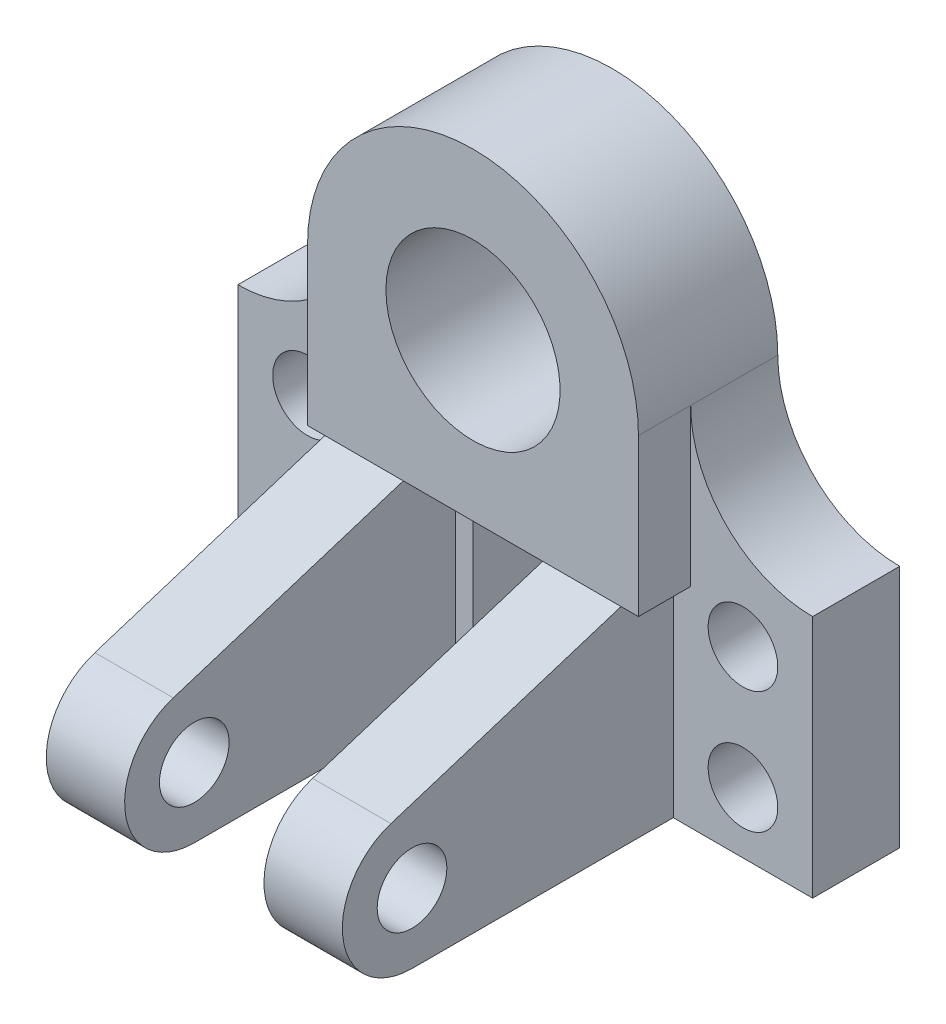
ISO-10303-21;
HEADER;
FILE_DESCRIPTION(('STEP AP214'),'2;1');
FILE_NAME('part.step','',(''),(''),'','','');
FILE_SCHEMA(('AUTOMOTIVE_DESIGN { 1 0 10303 214 1 1 1 1 }'));
ENDSEC;
DATA;
#1=APPLICATION_CONTEXT('core data for automotive mechanical design processes');
#2=APPLICATION_PROTOCOL_DEFINITION('international standard','automotive_design',2000,#1);
#3=PRODUCT_CONTEXT('',#1,'mechanical');
#4=PRODUCT('Part','Part','',(#3));
#5=PRODUCT_RELATED_PRODUCT_CATEGORY('part','',(#4));
#6=PRODUCT_DEFINITION_FORMATION('','',#4);
#7=PRODUCT_DEFINITION_CONTEXT('part definition',#1,'design');
#8=PRODUCT_DEFINITION('design','',#6,#7);
#9=PRODUCT_DEFINITION_SHAPE('','',#8);
#10=(LENGTH_UNIT() NAMED_UNIT(*) SI_UNIT(.MILLI.,.METRE.));
#11=(NAMED_UNIT(*) PLANE_ANGLE_UNIT() SI_UNIT($,.RADIAN.));
#12=(NAMED_UNIT(*) SI_UNIT($,.STERADIAN.) SOLID_ANGLE_UNIT());
#13=UNCERTAINTY_MEASURE_WITH_UNIT(LENGTH_MEASURE(1.E-05),#10,'distance_accuracy_value','');
#14=(GEOMETRIC_REPRESENTATION_CONTEXT(3) GLOBAL_UNCERTAINTY_ASSIGNED_CONTEXT((#13)) GLOBAL_UNIT_ASSIGNED_CONTEXT((#10,
#11,#12)) REPRESENTATION_CONTEXT('',''));
#15=CARTESIAN_POINT('',(0.,0.,0.));
#16=DIRECTION('',(0.,0.,1.));
#17=DIRECTION('',(1.,0.,0.));
#18=AXIS2_PLACEMENT_3D('',#15,#16,#17);
#19=CARTESIAN_POINT('',(-16.,-22.0813008130081,76.));
#20=DIRECTION('',(-1.,0.,0.));
#21=DIRECTION('',(0.,0.,1.));
#22=AXIS2_PLACEMENT_3D('',#19,#20,#21);
#23=PLANE('',#22);
#24=CARTESIAN_POINT('',(-16.,-6.08130081300815,60.));
#25=DIRECTION('',(-1.,0.,0.));
#26=DIRECTION('',(0.,0.,1.));
#27=AXIS2_PLACEMENT_3D('',#24,#25,#26);
#28=CIRCLE('',#27,8.00000000000001);
#29=CARTESIAN_POINT('',(-16.,-6.08130081300815,68.));
#30=VERTEX_POINT('',#29);
#31=EDGE_CURVE('E254',#30,#30,#28,.T.);
#32=ORIENTED_EDGE('',*,*,#31,.T.);
#33=EDGE_LOOP('',(#32));
#34=FACE_BOUND('',#33,.T.);
#35=CARTESIAN_POINT('',(-16.,-6.08130081300815,60.));
#36=DIRECTION('',(-1.,0.,0.));
#37=DIRECTION('',(0.,0.,1.));
#38=AXIS2_PLACEMENT_3D('',#35,#36,#37);
#39=CIRCLE('',#38,16.);
#40=CARTESIAN_POINT('',(-16.,-22.0813008130081,60.));
#41=VERTEX_POINT('',#40);
#42=CARTESIAN_POINT('',(-16.,9.17076668903895,64.8347116680314));
#43=VERTEX_POINT('',#42);
#44=EDGE_CURVE('E518',#41,#43,#39,.T.);
#45=ORIENTED_EDGE('',*,*,#44,.F.);
#46=DIRECTION('',(0.,0.,-1.));
#47=VECTOR('',#46,1.);
#48=CARTESIAN_POINT('',(-16.,-22.0813008130081,76.));
#49=LINE('',#48,#47);
#50=CARTESIAN_POINT('',(-16.,-22.0813008130081,0.));
#51=VERTEX_POINT('',#50);
#52=EDGE_CURVE('E112',#41,#51,#49,.T.);
#53=ORIENTED_EDGE('',*,*,#52,.T.);
#54=DIRECTION('',(0.,1.,0.));
#55=VECTOR('',#54,1.);
#56=CARTESIAN_POINT('',(-16.,-22.0813008130081,0.));
#57=LINE('',#56,#55);
#58=CARTESIAN_POINT('',(-16.,25.9186991869919,0.));
#59=VERTEX_POINT('',#58);
#60=EDGE_CURVE('E447',#51,#59,#57,.T.);
#61=ORIENTED_EDGE('',*,*,#60,.T.);
#62=DIRECTION('',(0.,0.,-1.));
#63=VECTOR('',#62,1.);
#64=CARTESIAN_POINT('',(-16.,25.9186991869919,76.));
#65=LINE('',#64,#63);
#66=CARTESIAN_POINT('',(-16.,25.9186991869919,12.));
#67=VERTEX_POINT('',#66);
#68=EDGE_CURVE('E271',#67,#59,#65,.T.);
#69=ORIENTED_EDGE('',*,*,#68,.F.);
#70=DIRECTION('',(0.,-0.302169479251962,0.953254218877943));
#71=VECTOR('',#70,1.);
#72=CARTESIAN_POINT('',(-16.,3.10115508736718,83.9825186555783));
#73=LINE('',#72,#71);
#74=EDGE_CURVE('E513',#67,#43,#73,.T.);
#75=ORIENTED_EDGE('',*,*,#74,.T.);
#76=EDGE_LOOP('',(#45,#53,#61,#69,#75));
#77=FACE_BOUND('',#76,.T.);
#78=ADVANCED_FACE('F87',(#34,#77),#23,.F.);
#79=CARTESIAN_POINT('',(-34.,-22.0813008130081,76.));
#80=DIRECTION('',(1.,0.,0.));
#81=DIRECTION('',(0.,0.,-1.));
#82=AXIS2_PLACEMENT_3D('',#79,#80,#81);
#83=PLANE('',#82);
#84=CARTESIAN_POINT('',(-34.,-6.08130081300815,60.));
#85=DIRECTION('',(-1.,0.,0.));
#86=DIRECTION('',(0.,0.,1.));
#87=AXIS2_PLACEMENT_3D('',#84,#85,#86);
#88=CIRCLE('',#87,8.00000000000001);
#89=CARTESIAN_POINT('',(-34.,-6.08130081300815,68.));
#90=VERTEX_POINT('',#89);
#91=EDGE_CURVE('E263',#90,#90,#88,.T.);
#92=ORIENTED_EDGE('',*,*,#91,.F.);
#93=EDGE_LOOP('',(#92));
#94=FACE_BOUND('',#93,.T.);
#95=DIRECTION('',(0.,0.,-1.));
#96=VECTOR('',#95,1.);
#97=CARTESIAN_POINT('',(-34.,-22.0813008130081,76.));
#98=LINE('',#97,#96);
#99=CARTESIAN_POINT('',(-34.,-22.0813008130081,60.));
#100=VERTEX_POINT('',#99);
#101=CARTESIAN_POINT('',(-34.,-22.0813008130081,0.));
#102=VERTEX_POINT('',#101);
#103=EDGE_CURVE('E257',#100,#102,#98,.T.);
#104=ORIENTED_EDGE('',*,*,#103,.F.);
#105=CARTESIAN_POINT('',(-34.,-6.08130081300815,60.));
#106=DIRECTION('',(-1.,0.,0.));
#107=DIRECTION('',(0.,0.,1.));
#108=AXIS2_PLACEMENT_3D('',#105,#106,#107);
#109=CIRCLE('',#108,16.);
#110=CARTESIAN_POINT('',(-34.,9.17076668903895,64.8347116680314));
#111=VERTEX_POINT('',#110);
#112=EDGE_CURVE('E241',#100,#111,#109,.T.);
#113=ORIENTED_EDGE('',*,*,#112,.T.);
#114=DIRECTION('',(0.,-0.302169479251962,0.953254218877943));
#115=VECTOR('',#114,1.);
#116=CARTESIAN_POINT('',(-34.,27.008688193053,8.5614110957514));
#117=LINE('',#116,#115);
#118=CARTESIAN_POINT('',(-34.,25.9186991869919,12.));
#119=VERTEX_POINT('',#118);
#120=EDGE_CURVE('E255',#119,#111,#117,.T.);
#121=ORIENTED_EDGE('',*,*,#120,.F.);
#122=DIRECTION('',(0.,0.,-1.));
#123=VECTOR('',#122,1.);
#124=CARTESIAN_POINT('',(-34.,25.9186991869919,76.));
#125=LINE('',#124,#123);
#126=CARTESIAN_POINT('',(-34.,25.9186991869919,0.));
#127=VERTEX_POINT('',#126);
#128=EDGE_CURVE('E267',#119,#127,#125,.T.);
#129=ORIENTED_EDGE('',*,*,#128,.T.);
#130=DIRECTION('',(0.,-1.,0.));
#131=VECTOR('',#130,1.);
#132=CARTESIAN_POINT('',(-34.,-22.0813008130081,0.));
#133=LINE('',#132,#131);
#134=EDGE_CURVE('E268',#127,#102,#133,.T.);
#135=ORIENTED_EDGE('',*,*,#134,.T.);
#136=EDGE_LOOP('',(#104,#113,#121,#129,#135));
#137=FACE_BOUND('',#136,.T.);
#138=ADVANCED_FACE('F266',(#94,#137),#83,.F.);
#139=CARTESIAN_POINT('',(16.,-22.0813008130081,76.));
#140=DIRECTION('',(-1.,0.,0.));
#141=DIRECTION('',(0.,0.,1.));
#142=AXIS2_PLACEMENT_3D('',#139,#140,#141);
#143=PLANE('',#142);
#144=CARTESIAN_POINT('',(16.,-6.08130081300815,60.));
#145=DIRECTION('',(-1.,0.,0.));
#146=DIRECTION('',(0.,0.,1.));
#147=AXIS2_PLACEMENT_3D('',#144,#145,#146);
#148=CIRCLE('',#147,8.00000000000001);
#149=CARTESIAN_POINT('',(16.,-6.08130081300815,68.));
#150=VERTEX_POINT('',#149);
#151=EDGE_CURVE('E529',#150,#150,#148,.T.);
#152=ORIENTED_EDGE('',*,*,#151,.F.);
#153=EDGE_LOOP('',(#152));
#154=FACE_BOUND('',#153,.T.);
#155=DIRECTION('',(0.,0.,-1.));
#156=VECTOR('',#155,1.);
#157=CARTESIAN_POINT('',(16.,-22.0813008130081,76.));
#158=LINE('',#157,#156);
#159=CARTESIAN_POINT('',(16.,-22.0813008130081,60.));
#160=VERTEX_POINT('',#159);
#161=CARTESIAN_POINT('',(16.,-22.0813008130081,0.));
#162=VERTEX_POINT('',#161);
#163=EDGE_CURVE('E449',#160,#162,#158,.T.);
#164=ORIENTED_EDGE('',*,*,#163,.F.);
#165=CARTESIAN_POINT('',(16.,-6.08130081300815,60.));
#166=DIRECTION('',(-1.,0.,0.));
#167=DIRECTION('',(0.,0.,1.));
#168=AXIS2_PLACEMENT_3D('',#165,#166,#167);
#169=CIRCLE('',#168,16.);
#170=CARTESIAN_POINT('',(16.,9.17076668903895,64.8347116680314));
#171=VERTEX_POINT('',#170);
#172=EDGE_CURVE('E522',#160,#171,#169,.T.);
#173=ORIENTED_EDGE('',*,*,#172,.T.);
#174=DIRECTION('',(0.,-0.302169479251962,0.953254218877943));
#175=VECTOR('',#174,1.);
#176=CARTESIAN_POINT('',(16.,3.10115508736718,83.9825186555783));
#177=LINE('',#176,#175);
#178=CARTESIAN_POINT('',(16.,25.9186991869919,12.));
#179=VERTEX_POINT('',#178);
#180=EDGE_CURVE('E517',#179,#171,#177,.T.);
#181=ORIENTED_EDGE('',*,*,#180,.F.);
#182=DIRECTION('',(0.,0.,-1.));
#183=VECTOR('',#182,1.);
#184=CARTESIAN_POINT('',(16.,25.9186991869919,76.));
#185=LINE('',#184,#183);
#186=CARTESIAN_POINT('',(16.,25.9186991869919,0.));
#187=VERTEX_POINT('',#186);
#188=EDGE_CURVE('E436',#179,#187,#185,.T.);
#189=ORIENTED_EDGE('',*,*,#188,.T.);
#190=DIRECTION('',(0.,1.,0.));
#191=VECTOR('',#190,1.);
#192=CARTESIAN_POINT('',(16.,-22.0813008130081,0.));
#193=LINE('',#192,#191);
#194=EDGE_CURVE('E483',#162,#187,#193,.T.);
#195=ORIENTED_EDGE('',*,*,#194,.F.);
#196=EDGE_LOOP('',(#164,#173,#181,#189,#195));
#197=FACE_BOUND('',#196,.T.);
#198=ADVANCED_FACE('F539',(#154,#197),#143,.T.);
#199=CARTESIAN_POINT('',(34.,-22.0813008130081,76.));
#200=DIRECTION('',(1.,0.,0.));
#201=DIRECTION('',(0.,0.,-1.));
#202=AXIS2_PLACEMENT_3D('',#199,#200,#201);
#203=PLANE('',#202);
#204=CARTESIAN_POINT('',(34.,-6.08130081300815,60.));
#205=DIRECTION('',(1.,0.,0.));
#206=DIRECTION('',(0.,0.,-1.));
#207=AXIS2_PLACEMENT_3D('',#204,#205,#206);
#208=CIRCLE('',#207,8.00000000000001);
#209=CARTESIAN_POINT('',(34.,-6.08130081300815,52.));
#210=VERTEX_POINT('',#209);
#211=EDGE_CURVE('E93',#210,#210,#208,.T.);
#212=ORIENTED_EDGE('',*,*,#211,.F.);
#213=EDGE_LOOP('',(#212));
#214=FACE_BOUND('',#213,.T.);
#215=CARTESIAN_POINT('',(34.,-6.08130081300815,60.));
#216=DIRECTION('',(1.,0.,0.));
#217=DIRECTION('',(0.,0.,-1.));
#218=AXIS2_PLACEMENT_3D('',#215,#216,#217);
#219=CIRCLE('',#218,16.);
#220=CARTESIAN_POINT('',(34.,9.17076668903895,64.8347116680314));
#221=VERTEX_POINT('',#220);
#222=CARTESIAN_POINT('',(34.,-22.0813008130081,60.));
#223=VERTEX_POINT('',#222);
#224=EDGE_CURVE('E525',#221,#223,#219,.T.);
#225=ORIENTED_EDGE('',*,*,#224,.T.);
#226=DIRECTION('',(0.,0.,-1.));
#227=VECTOR('',#226,1.);
#228=CARTESIAN_POINT('',(34.,-22.0813008130081,76.));
#229=LINE('',#228,#227);
#230=CARTESIAN_POINT('',(34.,-22.0813008130081,0.));
#231=VERTEX_POINT('',#230);
#232=EDGE_CURVE('E103',#223,#231,#229,.T.);
#233=ORIENTED_EDGE('',*,*,#232,.T.);
#234=DIRECTION('',(0.,-1.,0.));
#235=VECTOR('',#234,1.);
#236=CARTESIAN_POINT('',(34.,-22.0813008130081,0.));
#237=LINE('',#236,#235);
#238=CARTESIAN_POINT('',(34.,25.9186991869919,0.));
#239=VERTEX_POINT('',#238);
#240=EDGE_CURVE('E433',#239,#231,#237,.T.);
#241=ORIENTED_EDGE('',*,*,#240,.F.);
#242=DIRECTION('',(0.,0.,-1.));
#243=VECTOR('',#242,1.);
#244=CARTESIAN_POINT('',(34.,25.9186991869919,76.));
#245=LINE('',#244,#243);
#246=CARTESIAN_POINT('',(34.,25.9186991869919,12.));
#247=VERTEX_POINT('',#246);
#248=EDGE_CURVE('E431',#247,#239,#245,.T.);
#249=ORIENTED_EDGE('',*,*,#248,.F.);
#250=DIRECTION('',(0.,0.302169479251962,-0.953254218877943));
#251=VECTOR('',#250,1.);
#252=CARTESIAN_POINT('',(34.,3.10115508736718,83.9825186555783));
#253=LINE('',#252,#251);
#254=EDGE_CURVE('E96',#221,#247,#253,.T.);
#255=ORIENTED_EDGE('',*,*,#254,.F.);
#256=EDGE_LOOP('',(#225,#233,#241,#249,#255));
#257=FACE_BOUND('',#256,.T.);
#258=ADVANCED_FACE('F435',(#214,#257),#203,.T.);
#259=CARTESIAN_POINT('',(-66.,-22.0813008130081,-20.));
#260=DIRECTION('',(0.,-1.,0.));
#261=DIRECTION('',(0.,0.,-1.));
#262=AXIS2_PLACEMENT_3D('',#259,#260,#261);
#263=PLANE('',#262);
#264=ORIENTED_EDGE('',*,*,#52,.F.);
#265=DIRECTION('',(-1.,0.,0.));
#266=VECTOR('',#265,1.);
#267=CARTESIAN_POINT('',(42.,-22.0813008130081,60.));
#268=LINE('',#267,#266);
#269=EDGE_CURVE('E247',#41,#100,#268,.T.);
#270=ORIENTED_EDGE('',*,*,#269,.T.);
#271=ORIENTED_EDGE('',*,*,#103,.T.);
#272=DIRECTION('',(1.,0.,0.));
#273=VECTOR('',#272,1.);
#274=CARTESIAN_POINT('',(-66.,-22.0813008130081,0.));
#275=LINE('',#274,#273);
#276=CARTESIAN_POINT('',(-66.,-22.0813008130081,0.));
#277=VERTEX_POINT('',#276);
#278=EDGE_CURVE('E403',#277,#102,#275,.T.);
#279=ORIENTED_EDGE('',*,*,#278,.F.);
#280=DIRECTION('',(0.,0.,1.));
#281=VECTOR('',#280,1.);
#282=CARTESIAN_POINT('',(-66.,-22.0813008130081,-20.));
#283=LINE('',#282,#281);
#284=CARTESIAN_POINT('',(-66.,-22.0813008130081,-20.));
#285=VERTEX_POINT('',#284);
#286=EDGE_CURVE('E405',#285,#277,#283,.T.);
#287=ORIENTED_EDGE('',*,*,#286,.F.);
#288=DIRECTION('',(1.,0.,0.));
#289=VECTOR('',#288,1.);
#290=CARTESIAN_POINT('',(-66.,-22.0813008130081,-20.));
#291=LINE('',#290,#289);
#292=CARTESIAN_POINT('',(-12.,-22.0813008130081,-20.));
#293=VERTEX_POINT('',#292);
#294=EDGE_CURVE('E393',#285,#293,#291,.T.);
#295=ORIENTED_EDGE('',*,*,#294,.T.);
#296=DIRECTION('',(0.,0.,1.));
#297=VECTOR('',#296,1.);
#298=CARTESIAN_POINT('',(-12.,-22.0813008130081,-20.));
#299=LINE('',#298,#297);
#300=CARTESIAN_POINT('',(-12.,-22.0813008130081,0.));
#301=VERTEX_POINT('',#300);
#302=EDGE_CURVE('E406',#293,#301,#299,.T.);
#303=ORIENTED_EDGE('',*,*,#302,.T.);
#304=EDGE_CURVE('E404',#51,#301,#275,.T.);
#305=ORIENTED_EDGE('',*,*,#304,.F.);
#306=EDGE_LOOP('',(#264,#270,#271,#279,#287,#295,#303,#305));
#307=FACE_BOUND('',#306,.T.);
#308=ADVANCED_FACE('F256',(#307),#263,.T.);
#309=CARTESIAN_POINT('',(66.,-22.0813008130081,-20.));
#310=DIRECTION('',(0.,-1.,0.));
#311=DIRECTION('',(0.,0.,-1.));
#312=AXIS2_PLACEMENT_3D('',#309,#310,#311);
#313=PLANE('',#312);
#314=ORIENTED_EDGE('',*,*,#232,.F.);
#315=DIRECTION('',(-1.,0.,0.));
#316=VECTOR('',#315,1.);
#317=CARTESIAN_POINT('',(42.,-22.0813008130081,60.));
#318=LINE('',#317,#316);
#319=EDGE_CURVE('E12',#223,#160,#318,.T.);
#320=ORIENTED_EDGE('',*,*,#319,.T.);
#321=ORIENTED_EDGE('',*,*,#163,.T.);
#322=DIRECTION('',(1.,0.,0.));
#323=VECTOR('',#322,1.);
#324=CARTESIAN_POINT('',(66.,-22.0813008130081,0.));
#325=LINE('',#324,#323);
#326=CARTESIAN_POINT('',(12.,-22.0813008130081,0.));
#327=VERTEX_POINT('',#326);
#328=EDGE_CURVE('E310',#327,#162,#325,.T.);
#329=ORIENTED_EDGE('',*,*,#328,.F.);
#330=DIRECTION('',(0.,0.,1.));
#331=VECTOR('',#330,1.);
#332=CARTESIAN_POINT('',(12.,-22.0813008130081,-20.));
#333=LINE('',#332,#331);
#334=CARTESIAN_POINT('',(12.,-22.0813008130081,-20.));
#335=VERTEX_POINT('',#334);
#336=EDGE_CURVE('E314',#335,#327,#333,.T.);
#337=ORIENTED_EDGE('',*,*,#336,.F.);
#338=DIRECTION('',(1.,0.,0.));
#339=VECTOR('',#338,1.);
#340=CARTESIAN_POINT('',(66.,-22.0813008130081,-20.));
#341=LINE('',#340,#339);
#342=CARTESIAN_POINT('',(66.,-22.0813008130081,-20.));
#343=VERTEX_POINT('',#342);
#344=EDGE_CURVE('E313',#335,#343,#341,.T.);
#345=ORIENTED_EDGE('',*,*,#344,.T.);
#346=DIRECTION('',(0.,0.,1.));
#347=VECTOR('',#346,1.);
#348=CARTESIAN_POINT('',(66.,-22.0813008130081,-20.));
#349=LINE('',#348,#347);
#350=CARTESIAN_POINT('',(66.,-22.0813008130081,0.));
#351=VERTEX_POINT('',#350);
#352=EDGE_CURVE('E325',#343,#351,#349,.T.);
#353=ORIENTED_EDGE('',*,*,#352,.T.);
#354=EDGE_CURVE('E317',#231,#351,#325,.T.);
#355=ORIENTED_EDGE('',*,*,#354,.F.);
#356=EDGE_LOOP('',(#314,#320,#321,#329,#337,#345,#353,#355));
#357=FACE_BOUND('',#356,.T.);
#358=ADVANCED_FACE('F512',(#357),#313,.T.);
#359=CARTESIAN_POINT('',(-38.,25.9186991869919,12.));
#360=DIRECTION('',(0.,-1.,0.));
#361=DIRECTION('',(1.,0.,0.));
#362=AXIS2_PLACEMENT_3D('',#359,#360,#361);
#363=PLANE('',#362);
#364=ORIENTED_EDGE('',*,*,#188,.F.);
#365=DIRECTION('',(-1.,0.,0.));
#366=VECTOR('',#365,1.);
#367=CARTESIAN_POINT('',(-38.,25.9186991869919,12.));
#368=LINE('',#367,#366);
#369=EDGE_CURVE('E357',#179,#67,#368,.T.);
#370=ORIENTED_EDGE('',*,*,#369,.T.);
#371=ORIENTED_EDGE('',*,*,#68,.T.);
#372=DIRECTION('',(1.,0.,0.));
#373=VECTOR('',#372,1.);
#374=CARTESIAN_POINT('',(0.,25.9186991869919,0.));
#375=LINE('',#374,#373);
#376=CARTESIAN_POINT('',(-12.,25.9186991869919,0.));
#377=VERTEX_POINT('',#376);
#378=EDGE_CURVE('E412',#59,#377,#375,.T.);
#379=ORIENTED_EDGE('',*,*,#378,.T.);
#380=DIRECTION('',(0.,0.,-1.));
#381=VECTOR('',#380,1.);
#382=CARTESIAN_POINT('',(-12.,25.9186991869919,-20.));
#383=LINE('',#382,#381);
#384=CARTESIAN_POINT('',(-12.,25.9186991869919,-20.));
#385=VERTEX_POINT('',#384);
#386=EDGE_CURVE('E366',#377,#385,#383,.T.);
#387=ORIENTED_EDGE('',*,*,#386,.T.);
#388=DIRECTION('',(-1.,0.,0.));
#389=VECTOR('',#388,1.);
#390=CARTESIAN_POINT('',(-38.,25.9186991869919,-20.));
#391=LINE('',#390,#389);
#392=CARTESIAN_POINT('',(12.,25.9186991869918,-20.));
#393=VERTEX_POINT('',#392);
#394=EDGE_CURVE('E349',#393,#385,#391,.T.);
#395=ORIENTED_EDGE('',*,*,#394,.F.);
#396=DIRECTION('',(0.,0.,-1.));
#397=VECTOR('',#396,1.);
#398=CARTESIAN_POINT('',(12.,25.9186991869919,12.));
#399=LINE('',#398,#397);
#400=CARTESIAN_POINT('',(12.,25.9186991869918,0.));
#401=VERTEX_POINT('',#400);
#402=EDGE_CURVE('E337',#401,#393,#399,.T.);
#403=ORIENTED_EDGE('',*,*,#402,.F.);
#404=DIRECTION('',(1.,0.,0.));
#405=VECTOR('',#404,1.);
#406=CARTESIAN_POINT('',(-38.,25.9186991869919,0.));
#407=LINE('',#406,#405);
#408=EDGE_CURVE('E332',#401,#187,#407,.T.);
#409=ORIENTED_EDGE('',*,*,#408,.T.);
#410=EDGE_LOOP('',(#364,#370,#371,#379,#387,#395,#403,#409));
#411=FACE_BOUND('',#410,.T.);
#412=ADVANCED_FACE('F478',(#411),#363,.T.);
#413=CARTESIAN_POINT('',(0.,0.,0.));
#414=DIRECTION('',(0.,0.,-1.));
#415=DIRECTION('',(-1.,0.,0.));
#416=AXIS2_PLACEMENT_3D('',#413,#414,#415);
#417=PLANE('',#416);
#418=ORIENTED_EDGE('',*,*,#328,.T.);
#419=ORIENTED_EDGE('',*,*,#194,.T.);
#420=ORIENTED_EDGE('',*,*,#408,.F.);
#421=DIRECTION('',(0.,-1.,0.));
#422=VECTOR('',#421,1.);
#423=CARTESIAN_POINT('',(12.,-22.0813008130081,0.));
#424=LINE('',#423,#422);
#425=EDGE_CURVE('E320',#401,#327,#424,.T.);
#426=ORIENTED_EDGE('',*,*,#425,.T.);
#427=EDGE_LOOP('',(#418,#419,#420,#426));
#428=FACE_BOUND('',#427,.T.);
#429=ADVANCED_FACE('F514',(#428),#417,.F.);
#430=CARTESIAN_POINT('',(0.,0.,0.));
#431=DIRECTION('',(0.,0.,1.));
#432=DIRECTION('',(1.,0.,0.));
#433=AXIS2_PLACEMENT_3D('',#430,#431,#432);
#434=PLANE('',#433);
#435=ORIENTED_EDGE('',*,*,#378,.F.);
#436=ORIENTED_EDGE('',*,*,#60,.F.);
#437=ORIENTED_EDGE('',*,*,#304,.T.);
#438=DIRECTION('',(0.,1.,0.));
#439=VECTOR('',#438,1.);
#440=CARTESIAN_POINT('',(-12.,-22.0813008130081,0.));
#441=LINE('',#440,#439);
#442=EDGE_CURVE('E396',#301,#377,#441,.T.);
#443=ORIENTED_EDGE('',*,*,#442,.T.);
#444=EDGE_LOOP('',(#435,#436,#437,#443));
#445=FACE_BOUND('',#444,.T.);
#446=ADVANCED_FACE('F491',(#445),#434,.T.);
#447=CARTESIAN_POINT('',(-50.,-8.08130081300814,0.));
#448=DIRECTION('',(0.,0.,1.));
#449=DIRECTION('',(1.,0.,0.));
#450=AXIS2_PLACEMENT_3D('',#447,#448,#449);
#451=CIRCLE('',#450,8.);
#452=CARTESIAN_POINT('',(-42.,-8.08130081300814,0.));
#453=VERTEX_POINT('',#452);
#454=EDGE_CURVE('E379',#453,#453,#451,.T.);
#455=ORIENTED_EDGE('',*,*,#454,.F.);
#456=EDGE_LOOP('',(#455));
#457=FACE_BOUND('',#456,.T.);
#458=CARTESIAN_POINT('',(-50.,19.9186991869919,0.));
#459=DIRECTION('',(0.,0.,1.));
#460=DIRECTION('',(1.,0.,0.));
#461=AXIS2_PLACEMENT_3D('',#458,#459,#460);
#462=CIRCLE('',#461,8.);
#463=CARTESIAN_POINT('',(-42.,19.9186991869919,0.));
#464=VERTEX_POINT('',#463);
#465=EDGE_CURVE('E383',#464,#464,#462,.T.);
#466=ORIENTED_EDGE('',*,*,#465,.F.);
#467=EDGE_LOOP('',(#466));
#468=FACE_BOUND('',#467,.T.);
#469=ORIENTED_EDGE('',*,*,#278,.T.);
#470=ORIENTED_EDGE('',*,*,#134,.F.);
#471=CARTESIAN_POINT('',(-38.,25.9186991869919,0.));
#472=VERTEX_POINT('',#471);
#473=EDGE_CURVE('E415',#472,#127,#375,.T.);
#474=ORIENTED_EDGE('',*,*,#473,.F.);
#475=DIRECTION('',(0.,-1.,0.));
#476=VECTOR('',#475,1.);
#477=CARTESIAN_POINT('',(-38.,0.,0.));
#478=LINE('',#477,#476);
#479=CARTESIAN_POINT('',(-38.,61.9186991869919,0.));
#480=VERTEX_POINT('',#479);
#481=EDGE_CURVE('E416',#480,#472,#478,.T.);
#482=ORIENTED_EDGE('',*,*,#481,.F.);
#483=CARTESIAN_POINT('',(-66.,61.9186991869919,0.));
#484=DIRECTION('',(0.,0.,1.));
#485=DIRECTION('',(1.,0.,0.));
#486=AXIS2_PLACEMENT_3D('',#483,#484,#485);
#487=CIRCLE('',#486,28.);
#488=CARTESIAN_POINT('',(-66.,33.9186991869919,0.));
#489=VERTEX_POINT('',#488);
#490=EDGE_CURVE('E283',#480,#489,#487,.F.);
#491=ORIENTED_EDGE('',*,*,#490,.T.);
#492=DIRECTION('',(0.,-1.,0.));
#493=VECTOR('',#492,1.);
#494=CARTESIAN_POINT('',(-66.,61.9186991869919,0.));
#495=LINE('',#494,#493);
#496=EDGE_CURVE('E388',#489,#277,#495,.T.);
#497=ORIENTED_EDGE('',*,*,#496,.T.);
#498=EDGE_LOOP('',(#469,#470,#474,#482,#491,#497));
#499=FACE_BOUND('',#498,.T.);
#500=ADVANCED_FACE('F463',(#457,#468,#499),#434,.T.);
#501=ORIENTED_EDGE('',*,*,#248,.T.);
#502=CARTESIAN_POINT('',(38.,25.9186991869919,0.));
#503=VERTEX_POINT('',#502);
#504=EDGE_CURVE('E329',#239,#503,#407,.T.);
#505=ORIENTED_EDGE('',*,*,#504,.T.);
#506=DIRECTION('',(0.,0.,-1.));
#507=VECTOR('',#506,1.);
#508=CARTESIAN_POINT('',(38.,25.9186991869919,12.));
#509=LINE('',#508,#507);
#510=CARTESIAN_POINT('',(38.,25.9186991869919,12.));
#511=VERTEX_POINT('',#510);
#512=EDGE_CURVE('E373',#511,#503,#509,.T.);
#513=ORIENTED_EDGE('',*,*,#512,.F.);
#514=EDGE_CURVE('E355',#511,#247,#368,.T.);
#515=ORIENTED_EDGE('',*,*,#514,.T.);
#516=EDGE_LOOP('',(#501,#505,#513,#515));
#517=FACE_BOUND('',#516,.T.);
#518=ADVANCED_FACE('F446',(#517),#363,.T.);
#519=ORIENTED_EDGE('',*,*,#473,.T.);
#520=ORIENTED_EDGE('',*,*,#128,.F.);
#521=CARTESIAN_POINT('',(-38.,25.9186991869919,12.));
#522=VERTEX_POINT('',#521);
#523=EDGE_CURVE('E354',#119,#522,#368,.T.);
#524=ORIENTED_EDGE('',*,*,#523,.T.);
#525=DIRECTION('',(0.,0.,-1.));
#526=VECTOR('',#525,1.);
#527=CARTESIAN_POINT('',(-38.,25.9186991869919,12.));
#528=LINE('',#527,#526);
#529=EDGE_CURVE('E367',#522,#472,#528,.T.);
#530=ORIENTED_EDGE('',*,*,#529,.T.);
#531=EDGE_LOOP('',(#519,#520,#524,#530));
#532=FACE_BOUND('',#531,.T.);
#533=ADVANCED_FACE('F468',(#532),#363,.T.);
#534=CARTESIAN_POINT('',(-66.,61.9186991869919,-20.));
#535=DIRECTION('',(-1.,0.,0.));
#536=DIRECTION('',(0.,0.,1.));
#537=AXIS2_PLACEMENT_3D('',#534,#535,#536);
#538=PLANE('',#537);
#539=ORIENTED_EDGE('',*,*,#496,.F.);
#540=DIRECTION('',(0.,0.,1.));
#541=VECTOR('',#540,1.);
#542=CARTESIAN_POINT('',(-66.,33.9186991869919,-32.));
#543=LINE('',#542,#541);
#544=CARTESIAN_POINT('',(-66.,33.9186991869919,-20.));
#545=VERTEX_POINT('',#544);
#546=EDGE_CURVE('E289',#545,#489,#543,.T.);
#547=ORIENTED_EDGE('',*,*,#546,.F.);
#548=DIRECTION('',(0.,-1.,0.));
#549=VECTOR('',#548,1.);
#550=CARTESIAN_POINT('',(-66.,61.9186991869919,-20.));
#551=LINE('',#550,#549);
#552=EDGE_CURVE('E395',#545,#285,#551,.T.);
#553=ORIENTED_EDGE('',*,*,#552,.T.);
#554=ORIENTED_EDGE('',*,*,#286,.T.);
#555=EDGE_LOOP('',(#539,#547,#553,#554));
#556=FACE_BOUND('',#555,.T.);
#557=ADVANCED_FACE('F90',(#556),#538,.T.);
#558=CARTESIAN_POINT('',(0.,0.,-20.));
#559=DIRECTION('',(0.,0.,1.));
#560=DIRECTION('',(1.,0.,0.));
#561=AXIS2_PLACEMENT_3D('',#558,#559,#560);
#562=PLANE('',#561);
#563=CARTESIAN_POINT('',(50.,-8.08130081300814,-20.));
#564=DIRECTION('',(0.,0.,1.));
#565=DIRECTION('',(-1.,0.,0.));
#566=AXIS2_PLACEMENT_3D('',#563,#564,#565);
#567=CIRCLE('',#566,8.);
#568=CARTESIAN_POINT('',(42.,-8.08130081300814,-20.));
#569=VERTEX_POINT('',#568);
#570=EDGE_CURVE('E296',#569,#569,#567,.T.);
#571=ORIENTED_EDGE('',*,*,#570,.T.);
#572=EDGE_LOOP('',(#571));
#573=FACE_BOUND('',#572,.T.);
#574=CARTESIAN_POINT('',(50.,19.9186991869919,-20.));
#575=DIRECTION('',(0.,0.,1.));
#576=DIRECTION('',(-1.,0.,0.));
#577=AXIS2_PLACEMENT_3D('',#574,#575,#576);
#578=CIRCLE('',#577,8.);
#579=CARTESIAN_POINT('',(42.,19.9186991869919,-20.));
#580=VERTEX_POINT('',#579);
#581=EDGE_CURVE('E291',#580,#580,#578,.T.);
#582=ORIENTED_EDGE('',*,*,#581,.T.);
#583=EDGE_LOOP('',(#582));
#584=FACE_BOUND('',#583,.T.);
#585=CARTESIAN_POINT('',(-50.,19.9186991869919,-20.));
#586=DIRECTION('',(0.,0.,1.));
#587=DIRECTION('',(1.,0.,0.));
#588=AXIS2_PLACEMENT_3D('',#585,#586,#587);
#589=CIRCLE('',#588,8.);
#590=CARTESIAN_POINT('',(-42.,19.9186991869919,-20.));
#591=VERTEX_POINT('',#590);
#592=EDGE_CURVE('E390',#591,#591,#589,.T.);
#593=ORIENTED_EDGE('',*,*,#592,.T.);
#594=EDGE_LOOP('',(#593));
#595=FACE_BOUND('',#594,.T.);
#596=CARTESIAN_POINT('',(-50.,-8.08130081300814,-20.));
#597=DIRECTION('',(0.,0.,1.));
#598=DIRECTION('',(1.,0.,0.));
#599=AXIS2_PLACEMENT_3D('',#596,#597,#598);
#600=CIRCLE('',#599,8.);
#601=CARTESIAN_POINT('',(-42.,-8.08130081300814,-20.));
#602=VERTEX_POINT('',#601);
#603=EDGE_CURVE('E381',#602,#602,#600,.T.);
#604=ORIENTED_EDGE('',*,*,#603,.T.);
#605=EDGE_LOOP('',(#604));
#606=FACE_BOUND('',#605,.T.);
#607=CARTESIAN_POINT('',(0.,61.9186991869919,-20.));
#608=DIRECTION('',(0.,0.,-1.));
#609=DIRECTION('',(-1.,0.,0.));
#610=AXIS2_PLACEMENT_3D('',#607,#608,#609);
#611=CIRCLE('',#610,20.);
#612=CARTESIAN_POINT('',(-20.,61.9186991869919,-20.));
#613=VERTEX_POINT('',#612);
#614=EDGE_CURVE('E340',#613,#613,#611,.T.);
#615=ORIENTED_EDGE('',*,*,#614,.F.);
#616=EDGE_LOOP('',(#615));
#617=FACE_BOUND('',#616,.T.);
#618=CARTESIAN_POINT('',(0.,61.9186991869919,-20.));
#619=DIRECTION('',(0.,0.,-1.));
#620=DIRECTION('',(-1.,0.,0.));
#621=AXIS2_PLACEMENT_3D('',#618,#619,#620);
#622=CIRCLE('',#621,38.);
#623=CARTESIAN_POINT('',(-38.,61.9186991869919,-20.));
#624=VERTEX_POINT('',#623);
#625=CARTESIAN_POINT('',(38.,61.9186991869919,-20.));
#626=VERTEX_POINT('',#625);
#627=EDGE_CURVE('E342',#624,#626,#622,.T.);
#628=ORIENTED_EDGE('',*,*,#627,.T.);
#629=CARTESIAN_POINT('',(66.,61.9186991869919,-20.));
#630=DIRECTION('',(0.,0.,1.));
#631=DIRECTION('',(1.,0.,0.));
#632=AXIS2_PLACEMENT_3D('',#629,#630,#631);
#633=CIRCLE('',#632,28.);
#634=CARTESIAN_POINT('',(66.,33.9186991869919,-20.));
#635=VERTEX_POINT('',#634);
#636=EDGE_CURVE('E284',#626,#635,#633,.T.);
#637=ORIENTED_EDGE('',*,*,#636,.T.);
#638=DIRECTION('',(0.,1.,0.));
#639=VECTOR('',#638,1.);
#640=CARTESIAN_POINT('',(66.,61.9186991869919,-20.));
#641=LINE('',#640,#639);
#642=EDGE_CURVE('E305',#343,#635,#641,.T.);
#643=ORIENTED_EDGE('',*,*,#642,.F.);
#644=ORIENTED_EDGE('',*,*,#344,.F.);
#645=DIRECTION('',(0.,-1.,0.));
#646=VECTOR('',#645,1.);
#647=CARTESIAN_POINT('',(12.,-22.0813008130081,-20.));
#648=LINE('',#647,#646);
#649=EDGE_CURVE('E306',#393,#335,#648,.T.);
#650=ORIENTED_EDGE('',*,*,#649,.F.);
#651=ORIENTED_EDGE('',*,*,#394,.T.);
#652=DIRECTION('',(0.,1.,0.));
#653=VECTOR('',#652,1.);
#654=CARTESIAN_POINT('',(-12.,-22.0813008130081,-20.));
#655=LINE('',#654,#653);
#656=EDGE_CURVE('E398',#293,#385,#655,.T.);
#657=ORIENTED_EDGE('',*,*,#656,.F.);
#658=ORIENTED_EDGE('',*,*,#294,.F.);
#659=ORIENTED_EDGE('',*,*,#552,.F.);
#660=CARTESIAN_POINT('',(-66.,61.9186991869919,-20.));
#661=DIRECTION('',(0.,0.,1.));
#662=DIRECTION('',(1.,0.,0.));
#663=AXIS2_PLACEMENT_3D('',#660,#661,#662);
#664=CIRCLE('',#663,28.);
#665=EDGE_CURVE('E290',#624,#545,#664,.F.);
#666=ORIENTED_EDGE('',*,*,#665,.F.);
#667=EDGE_LOOP('',(#628,#637,#643,#644,#650,#651,#657,#658,#659,#666));
#668=FACE_BOUND('',#667,.T.);
#669=ADVANCED_FACE('F504',(#573,#584,#595,#606,#617,#668),#562,.F.);
#670=CARTESIAN_POINT('',(38.,25.9186991869919,12.));
#671=DIRECTION('',(1.,0.,0.));
#672=DIRECTION('',(0.,0.,-1.));
#673=AXIS2_PLACEMENT_3D('',#670,#671,#672);
#674=PLANE('',#673);
#675=ORIENTED_EDGE('',*,*,#512,.T.);
#676=DIRECTION('',(0.,1.,0.));
#677=VECTOR('',#676,1.);
#678=CARTESIAN_POINT('',(38.,25.9186991869919,0.));
#679=LINE('',#678,#677);
#680=CARTESIAN_POINT('',(38.,61.9186991869919,0.));
#681=VERTEX_POINT('',#680);
#682=EDGE_CURVE('E324',#503,#681,#679,.T.);
#683=ORIENTED_EDGE('',*,*,#682,.T.);
#684=DIRECTION('',(0.,0.,-1.));
#685=VECTOR('',#684,1.);
#686=CARTESIAN_POINT('',(38.,61.9186991869919,12.));
#687=LINE('',#686,#685);
#688=CARTESIAN_POINT('',(38.,61.9186991869919,12.));
#689=VERTEX_POINT('',#688);
#690=EDGE_CURVE('E363',#689,#681,#687,.T.);
#691=ORIENTED_EDGE('',*,*,#690,.F.);
#692=DIRECTION('',(0.,-1.,0.));
#693=VECTOR('',#692,1.);
#694=CARTESIAN_POINT('',(38.,25.9186991869919,12.));
#695=LINE('',#694,#693);
#696=EDGE_CURVE('E346',#689,#511,#695,.T.);
#697=ORIENTED_EDGE('',*,*,#696,.T.);
#698=EDGE_LOOP('',(#675,#683,#691,#697));
#699=FACE_BOUND('',#698,.T.);
#700=ADVANCED_FACE('F452',(#699),#674,.T.);
#701=CARTESIAN_POINT('',(-12.,-22.0813008130081,-20.));
#702=DIRECTION('',(1.,0.,0.));
#703=DIRECTION('',(0.,0.,-1.));
#704=AXIS2_PLACEMENT_3D('',#701,#702,#703);
#705=PLANE('',#704);
#706=ORIENTED_EDGE('',*,*,#386,.F.);
#707=ORIENTED_EDGE('',*,*,#442,.F.);
#708=ORIENTED_EDGE('',*,*,#302,.F.);
#709=ORIENTED_EDGE('',*,*,#656,.T.);
#710=EDGE_LOOP('',(#706,#707,#708,#709));
#711=FACE_BOUND('',#710,.T.);
#712=ADVANCED_FACE('F499',(#711),#705,.T.);
#713=CARTESIAN_POINT('',(-50.,19.9186991869919,-20.));
#714=DIRECTION('',(0.,0.,1.));
#715=DIRECTION('',(1.,0.,0.));
#716=AXIS2_PLACEMENT_3D('',#713,#714,#715);
#717=CYLINDRICAL_SURFACE('',#716,8.);
#718=ORIENTED_EDGE('',*,*,#592,.F.);
#719=EDGE_LOOP('',(#718));
#720=FACE_BOUND('',#719,.T.);
#721=ORIENTED_EDGE('',*,*,#465,.T.);
#722=EDGE_LOOP('',(#721));
#723=FACE_BOUND('',#722,.T.);
#724=ADVANCED_FACE('F597',(#720,#723),#717,.F.);
#725=CARTESIAN_POINT('',(-50.,-8.08130081300814,-20.));
#726=DIRECTION('',(0.,0.,1.));
#727=DIRECTION('',(1.,0.,0.));
#728=AXIS2_PLACEMENT_3D('',#725,#726,#727);
#729=CYLINDRICAL_SURFACE('',#728,8.);
#730=ORIENTED_EDGE('',*,*,#603,.F.);
#731=EDGE_LOOP('',(#730));
#732=FACE_BOUND('',#731,.T.);
#733=ORIENTED_EDGE('',*,*,#454,.T.);
#734=EDGE_LOOP('',(#733));
#735=FACE_BOUND('',#734,.T.);
#736=ADVANCED_FACE('F596',(#732,#735),#729,.F.);
#737=CARTESIAN_POINT('',(0.,61.9186991869919,12.));
#738=DIRECTION('',(0.,0.,-1.));
#739=DIRECTION('',(-1.,0.,0.));
#740=AXIS2_PLACEMENT_3D('',#737,#738,#739);
#741=CYLINDRICAL_SURFACE('',#740,38.);
#742=ORIENTED_EDGE('',*,*,#627,.F.);
#743=DIRECTION('',(0.,0.,-1.));
#744=VECTOR('',#743,1.);
#745=CARTESIAN_POINT('',(-38.,61.9186991869919,12.));
#746=LINE('',#745,#744);
#747=EDGE_CURVE('E369',#480,#624,#746,.T.);
#748=ORIENTED_EDGE('',*,*,#747,.F.);
#749=CARTESIAN_POINT('',(-38.,61.9186991869919,12.));
#750=VERTEX_POINT('',#749);
#751=EDGE_CURVE('E364',#750,#480,#746,.T.);
#752=ORIENTED_EDGE('',*,*,#751,.F.);
#753=CARTESIAN_POINT('',(0.,61.9186991869919,12.));
#754=DIRECTION('',(0.,0.,-1.));
#755=DIRECTION('',(-1.,0.,0.));
#756=AXIS2_PLACEMENT_3D('',#753,#754,#755);
#757=CIRCLE('',#756,38.);
#758=EDGE_CURVE('E345',#750,#689,#757,.T.);
#759=ORIENTED_EDGE('',*,*,#758,.T.);
#760=ORIENTED_EDGE('',*,*,#690,.T.);
#761=DIRECTION('',(0.,0.,1.));
#762=VECTOR('',#761,1.);
#763=CARTESIAN_POINT('',(38.,61.9186991869919,12.));
#764=LINE('',#763,#762);
#765=EDGE_CURVE('E331',#626,#681,#764,.T.);
#766=ORIENTED_EDGE('',*,*,#765,.F.);
#767=EDGE_LOOP('',(#742,#748,#752,#759,#760,#766));
#768=FACE_BOUND('',#767,.T.);
#769=ADVANCED_FACE('F457',(#768),#741,.T.);
#770=CARTESIAN_POINT('',(-38.,61.9186991869919,12.));
#771=DIRECTION('',(-1.,0.,0.));
#772=DIRECTION('',(0.,-1.,0.));
#773=AXIS2_PLACEMENT_3D('',#770,#771,#772);
#774=PLANE('',#773);
#775=ORIENTED_EDGE('',*,*,#751,.T.);
#776=ORIENTED_EDGE('',*,*,#481,.T.);
#777=ORIENTED_EDGE('',*,*,#529,.F.);
#778=DIRECTION('',(0.,1.,0.));
#779=VECTOR('',#778,1.);
#780=CARTESIAN_POINT('',(-38.,61.9186991869919,12.));
#781=LINE('',#780,#779);
#782=EDGE_CURVE('E356',#522,#750,#781,.T.);
#783=ORIENTED_EDGE('',*,*,#782,.T.);
#784=EDGE_LOOP('',(#775,#776,#777,#783));
#785=FACE_BOUND('',#784,.T.);
#786=ADVANCED_FACE('F462',(#785),#774,.T.);
#787=CARTESIAN_POINT('',(0.,61.9186991869919,12.));
#788=DIRECTION('',(0.,0.,-1.));
#789=DIRECTION('',(-1.,0.,0.));
#790=AXIS2_PLACEMENT_3D('',#787,#788,#789);
#791=PLANE('',#790);
#792=CARTESIAN_POINT('',(0.,61.9186991869919,12.));
#793=DIRECTION('',(0.,0.,-1.));
#794=DIRECTION('',(-1.,0.,0.));
#795=AXIS2_PLACEMENT_3D('',#792,#793,#794);
#796=CIRCLE('',#795,20.);
#797=CARTESIAN_POINT('',(-20.,61.9186991869919,12.));
#798=VERTEX_POINT('',#797);
#799=EDGE_CURVE('E336',#798,#798,#796,.T.);
#800=ORIENTED_EDGE('',*,*,#799,.T.);
#801=EDGE_LOOP('',(#800));
#802=FACE_BOUND('',#801,.T.);
#803=ORIENTED_EDGE('',*,*,#758,.F.);
#804=ORIENTED_EDGE('',*,*,#782,.F.);
#805=ORIENTED_EDGE('',*,*,#523,.F.);
#806=EDGE_CURVE('E359',#67,#119,#368,.T.);
#807=ORIENTED_EDGE('',*,*,#806,.F.);
#808=ORIENTED_EDGE('',*,*,#369,.F.);
#809=DIRECTION('',(1.,0.,0.));
#810=VECTOR('',#809,1.);
#811=CARTESIAN_POINT('',(0.,25.9186991869919,12.));
#812=LINE('',#811,#810);
#813=EDGE_CURVE('E426',#179,#247,#812,.T.);
#814=ORIENTED_EDGE('',*,*,#813,.T.);
#815=ORIENTED_EDGE('',*,*,#514,.F.);
#816=ORIENTED_EDGE('',*,*,#696,.F.);
#817=EDGE_LOOP('',(#803,#804,#805,#807,#808,#814,#815,#816));
#818=FACE_BOUND('',#817,.T.);
#819=ADVANCED_FACE('F445',(#802,#818),#791,.F.);
#820=CARTESIAN_POINT('',(0.,61.9186991869919,12.));
#821=DIRECTION('',(0.,0.,-1.));
#822=DIRECTION('',(-1.,0.,0.));
#823=AXIS2_PLACEMENT_3D('',#820,#821,#822);
#824=CYLINDRICAL_SURFACE('',#823,20.);
#825=ORIENTED_EDGE('',*,*,#614,.T.);
#826=EDGE_LOOP('',(#825));
#827=FACE_BOUND('',#826,.T.);
#828=ORIENTED_EDGE('',*,*,#799,.F.);
#829=EDGE_LOOP('',(#828));
#830=FACE_BOUND('',#829,.T.);
#831=ADVANCED_FACE('F580',(#827,#830),#824,.F.);
#832=CARTESIAN_POINT('',(66.,61.9186991869919,-20.));
#833=DIRECTION('',(1.,0.,0.));
#834=DIRECTION('',(0.,0.,-1.));
#835=AXIS2_PLACEMENT_3D('',#832,#833,#834);
#836=PLANE('',#835);
#837=DIRECTION('',(0.,0.,1.));
#838=VECTOR('',#837,1.);
#839=CARTESIAN_POINT('',(66.,33.9186991869919,-32.));
#840=LINE('',#839,#838);
#841=CARTESIAN_POINT('',(66.,33.9186991869919,0.));
#842=VERTEX_POINT('',#841);
#843=EDGE_CURVE('E276',#635,#842,#840,.T.);
#844=ORIENTED_EDGE('',*,*,#843,.T.);
#845=DIRECTION('',(0.,1.,0.));
#846=VECTOR('',#845,1.);
#847=CARTESIAN_POINT('',(66.,61.9186991869919,0.));
#848=LINE('',#847,#846);
#849=EDGE_CURVE('E302',#351,#842,#848,.T.);
#850=ORIENTED_EDGE('',*,*,#849,.F.);
#851=ORIENTED_EDGE('',*,*,#352,.F.);
#852=ORIENTED_EDGE('',*,*,#642,.T.);
#853=EDGE_LOOP('',(#844,#850,#851,#852));
#854=FACE_BOUND('',#853,.T.);
#855=ADVANCED_FACE('F577',(#854),#836,.T.);
#856=CARTESIAN_POINT('',(12.,-22.0813008130081,-20.));
#857=DIRECTION('',(-1.,0.,0.));
#858=DIRECTION('',(0.,0.,1.));
#859=AXIS2_PLACEMENT_3D('',#856,#857,#858);
#860=PLANE('',#859);
#861=ORIENTED_EDGE('',*,*,#425,.F.);
#862=ORIENTED_EDGE('',*,*,#402,.T.);
#863=ORIENTED_EDGE('',*,*,#649,.T.);
#864=ORIENTED_EDGE('',*,*,#336,.T.);
#865=EDGE_LOOP('',(#861,#862,#863,#864));
#866=FACE_BOUND('',#865,.T.);
#867=ADVANCED_FACE('F509',(#866),#860,.T.);
#868=ORIENTED_EDGE('',*,*,#504,.F.);
#869=ORIENTED_EDGE('',*,*,#240,.T.);
#870=ORIENTED_EDGE('',*,*,#354,.T.);
#871=ORIENTED_EDGE('',*,*,#849,.T.);
#872=CARTESIAN_POINT('',(66.,61.9186991869919,0.));
#873=DIRECTION('',(0.,0.,-1.));
#874=DIRECTION('',(-1.,0.,0.));
#875=AXIS2_PLACEMENT_3D('',#872,#873,#874);
#876=CIRCLE('',#875,28.);
#877=EDGE_CURVE('E280',#681,#842,#876,.F.);
#878=ORIENTED_EDGE('',*,*,#877,.F.);
#879=ORIENTED_EDGE('',*,*,#682,.F.);
#880=EDGE_LOOP('',(#868,#869,#870,#871,#878,#879));
#881=FACE_BOUND('',#880,.T.);
#882=CARTESIAN_POINT('',(50.,19.9186991869919,0.));
#883=DIRECTION('',(0.,0.,1.));
#884=DIRECTION('',(-1.,0.,0.));
#885=AXIS2_PLACEMENT_3D('',#882,#883,#884);
#886=CIRCLE('',#885,8.);
#887=CARTESIAN_POINT('',(42.,19.9186991869919,0.));
#888=VERTEX_POINT('',#887);
#889=EDGE_CURVE('E295',#888,#888,#886,.T.);
#890=ORIENTED_EDGE('',*,*,#889,.F.);
#891=EDGE_LOOP('',(#890));
#892=FACE_BOUND('',#891,.T.);
#893=CARTESIAN_POINT('',(50.,-8.08130081300814,0.));
#894=DIRECTION('',(0.,0.,1.));
#895=DIRECTION('',(-1.,0.,0.));
#896=AXIS2_PLACEMENT_3D('',#893,#894,#895);
#897=CIRCLE('',#896,8.);
#898=CARTESIAN_POINT('',(42.,-8.08130081300814,0.));
#899=VERTEX_POINT('',#898);
#900=EDGE_CURVE('E297',#899,#899,#897,.T.);
#901=ORIENTED_EDGE('',*,*,#900,.F.);
#902=EDGE_LOOP('',(#901));
#903=FACE_BOUND('',#902,.T.);
#904=ADVANCED_FACE('F566',(#881,#892,#903),#417,.F.);
#905=CARTESIAN_POINT('',(50.,-8.08130081300814,-20.));
#906=DIRECTION('',(0.,0.,1.));
#907=DIRECTION('',(1.,0.,0.));
#908=AXIS2_PLACEMENT_3D('',#905,#906,#907);
#909=CYLINDRICAL_SURFACE('',#908,8.);
#910=ORIENTED_EDGE('',*,*,#570,.F.);
#911=EDGE_LOOP('',(#910));
#912=FACE_BOUND('',#911,.T.);
#913=ORIENTED_EDGE('',*,*,#900,.T.);
#914=EDGE_LOOP('',(#913));
#915=FACE_BOUND('',#914,.T.);
#916=ADVANCED_FACE('F563',(#912,#915),#909,.F.);
#917=CARTESIAN_POINT('',(50.,19.9186991869919,-20.));
#918=DIRECTION('',(0.,0.,1.));
#919=DIRECTION('',(1.,0.,0.));
#920=AXIS2_PLACEMENT_3D('',#917,#918,#919);
#921=CYLINDRICAL_SURFACE('',#920,8.);
#922=ORIENTED_EDGE('',*,*,#581,.F.);
#923=EDGE_LOOP('',(#922));
#924=FACE_BOUND('',#923,.T.);
#925=ORIENTED_EDGE('',*,*,#889,.T.);
#926=EDGE_LOOP('',(#925));
#927=FACE_BOUND('',#926,.T.);
#928=ADVANCED_FACE('F558',(#924,#927),#921,.F.);
#929=CARTESIAN_POINT('',(-66.,61.9186991869919,-32.));
#930=DIRECTION('',(0.,0.,1.));
#931=DIRECTION('',(1.,0.,0.));
#932=AXIS2_PLACEMENT_3D('',#929,#930,#931);
#933=CYLINDRICAL_SURFACE('',#932,28.);
#934=ORIENTED_EDGE('',*,*,#665,.T.);
#935=ORIENTED_EDGE('',*,*,#546,.T.);
#936=ORIENTED_EDGE('',*,*,#490,.F.);
#937=ORIENTED_EDGE('',*,*,#747,.T.);
#938=EDGE_LOOP('',(#934,#935,#936,#937));
#939=FACE_BOUND('',#938,.T.);
#940=ADVANCED_FACE('F557',(#939),#933,.F.);
#941=CARTESIAN_POINT('',(66.,61.9186991869919,-32.));
#942=DIRECTION('',(0.,0.,1.));
#943=DIRECTION('',(1.,0.,0.));
#944=AXIS2_PLACEMENT_3D('',#941,#942,#943);
#945=CYLINDRICAL_SURFACE('',#944,28.);
#946=ORIENTED_EDGE('',*,*,#765,.T.);
#947=ORIENTED_EDGE('',*,*,#877,.T.);
#948=ORIENTED_EDGE('',*,*,#843,.F.);
#949=ORIENTED_EDGE('',*,*,#636,.F.);
#950=EDGE_LOOP('',(#946,#947,#948,#949));
#951=FACE_BOUND('',#950,.T.);
#952=ADVANCED_FACE('F555',(#951),#945,.F.);
#953=CARTESIAN_POINT('',(42.,-6.08130081300815,60.));
#954=DIRECTION('',(-1.,0.,0.));
#955=DIRECTION('',(0.,0.,1.));
#956=AXIS2_PLACEMENT_3D('',#953,#954,#955);
#957=CYLINDRICAL_SURFACE('',#956,16.);
#958=ORIENTED_EDGE('',*,*,#172,.F.);
#959=ORIENTED_EDGE('',*,*,#319,.F.);
#960=ORIENTED_EDGE('',*,*,#224,.F.);
#961=DIRECTION('',(-1.,0.,0.));
#962=VECTOR('',#961,1.);
#963=CARTESIAN_POINT('',(42.,9.17076668903895,64.8347116680314));
#964=LINE('',#963,#962);
#965=EDGE_CURVE('E427',#221,#171,#964,.T.);
#966=ORIENTED_EDGE('',*,*,#965,.T.);
#967=EDGE_LOOP('',(#958,#959,#960,#966));
#968=FACE_BOUND('',#967,.T.);
#969=ADVANCED_FACE('F553',(#968),#957,.T.);
#970=CARTESIAN_POINT('',(42.,27.008688193053,8.5614110957514));
#971=DIRECTION('',(0.,-0.953254218877943,-0.302169479251962));
#972=DIRECTION('',(0.,0.302169479251962,-0.953254218877943));
#973=AXIS2_PLACEMENT_3D('',#970,#971,#972);
#974=PLANE('',#973);
#975=ORIENTED_EDGE('',*,*,#180,.T.);
#976=ORIENTED_EDGE('',*,*,#965,.F.);
#977=ORIENTED_EDGE('',*,*,#254,.T.);
#978=ORIENTED_EDGE('',*,*,#813,.F.);
#979=EDGE_LOOP('',(#975,#976,#977,#978));
#980=FACE_BOUND('',#979,.T.);
#981=ADVANCED_FACE('F424',(#980),#974,.F.);
#982=ORIENTED_EDGE('',*,*,#806,.T.);
#983=ORIENTED_EDGE('',*,*,#120,.T.);
#984=EDGE_CURVE('E248',#43,#111,#964,.T.);
#985=ORIENTED_EDGE('',*,*,#984,.F.);
#986=ORIENTED_EDGE('',*,*,#74,.F.);
#987=EDGE_LOOP('',(#982,#983,#985,#986));
#988=FACE_BOUND('',#987,.T.);
#989=ADVANCED_FACE('F624',(#988),#974,.F.);
#990=ORIENTED_EDGE('',*,*,#44,.T.);
#991=ORIENTED_EDGE('',*,*,#984,.T.);
#992=ORIENTED_EDGE('',*,*,#112,.F.);
#993=ORIENTED_EDGE('',*,*,#269,.F.);
#994=EDGE_LOOP('',(#990,#991,#992,#993));
#995=FACE_BOUND('',#994,.T.);
#996=ADVANCED_FACE('F246',(#995),#957,.T.);
#997=CARTESIAN_POINT('',(42.,-6.08130081300815,60.));
#998=DIRECTION('',(-1.,0.,0.));
#999=DIRECTION('',(0.,0.,1.));
#1000=AXIS2_PLACEMENT_3D('',#997,#998,#999);
#1001=CYLINDRICAL_SURFACE('',#1000,8.00000000000001);
#1002=ORIENTED_EDGE('',*,*,#151,.T.);
#1003=EDGE_LOOP('',(#1002));
#1004=FACE_BOUND('',#1003,.T.);
#1005=ORIENTED_EDGE('',*,*,#211,.T.);
#1006=EDGE_LOOP('',(#1005));
#1007=FACE_BOUND('',#1006,.T.);
#1008=ADVANCED_FACE('F623',(#1004,#1007),#1001,.F.);
#1009=ORIENTED_EDGE('',*,*,#91,.T.);
#1010=EDGE_LOOP('',(#1009));
#1011=FACE_BOUND('',#1010,.T.);
#1012=ORIENTED_EDGE('',*,*,#31,.F.);
#1013=EDGE_LOOP('',(#1012));
#1014=FACE_BOUND('',#1013,.T.);
#1015=ADVANCED_FACE('F536',(#1011,#1014),#1001,.F.);
#1016=CLOSED_SHELL('',(#78,#138,#198,#258,#308,#358,#412,#429,#446,#500,#518,#533,#557,#669,
#700,#712,#724,#736,#769,#786,#819,#831,#855,#867,#904,#916,#928,#940,#952,#969,#981,#989,#996,
#1008,#1015));
#1017=MANIFOLD_SOLID_BREP('B2',#1016);
#1018=ADVANCED_BREP_SHAPE_REPRESENTATION('',(#18,#1017),#14);
#1019=SHAPE_DEFINITION_REPRESENTATION(#9,#1018);
ENDSEC;
END-ISO-10303-21;
